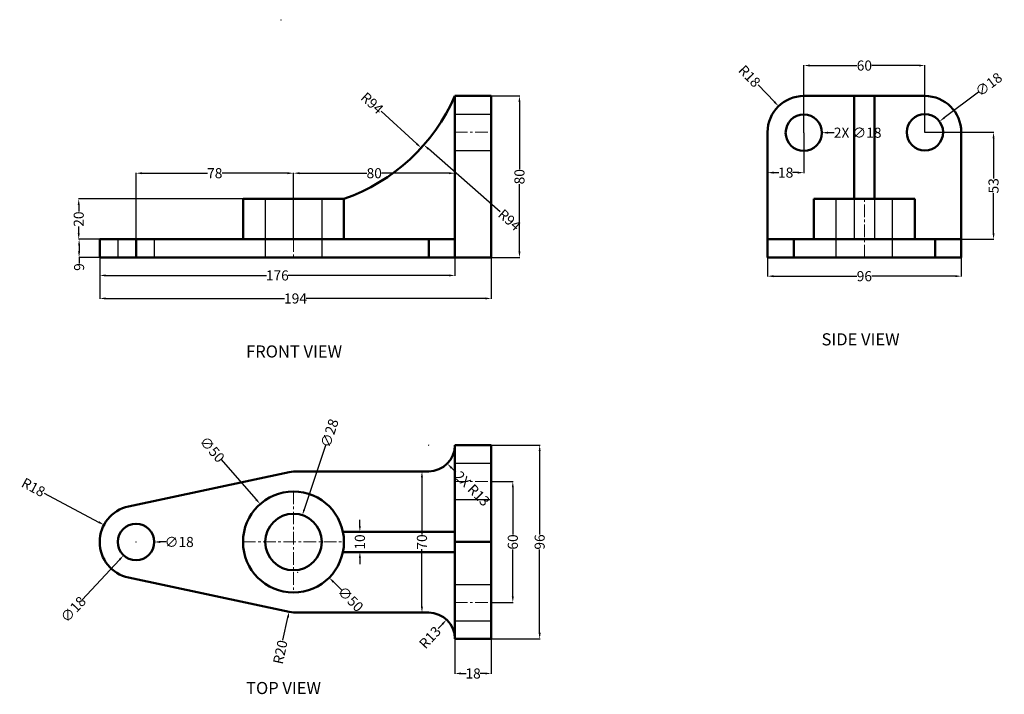
# Model space of a CAD drawing. Units: inches. Extents: x 93 to 580, y -115 to 220.
import ezdxf

# ---------------------------------------------------------------- set-up
doc = ezdxf.new("R2010")
doc.units = ezdxf.units.IN
doc.header["$MEASUREMENT"] = 0
doc.linetypes.add('CENTER', pattern=[2, 1.25, -0.25, 0.25, -0.25])
doc.linetypes.add('HIDDEN', pattern=[9.525, 6.35, -3.175])
for name, color, linetype, lineweight in [('M-CNTR', 1, 'CENTER', 18), ('M-DIMS', 2, 'Continuous', 25), ('M-HIDN', 3, 'HIDDEN', 25), ('M-OUTL', 7, 'Continuous', 50), ('M-TEXT', 7, 'Continuous', 25)]:
    doc.layers.add(name, color=color, linetype=linetype, lineweight=lineweight)
doc.styles.get("Standard").update_dxf_attribs({"font": 'arial.ttf'})
doc.dimstyles.get("Standard").update_dxf_attribs({"dimtxt": 5, "dimasz": 3, "dimexe": 0.18, "dimexo": 0.0625, "dimgap": 0.09, "dimtad": 0, "dimdec": 0, "dimzin": 0, "dimdsep": 46, "dimtxsty": 'Standard', "dimcen": 0.09, "dimadec": 0, "dimazin": 0, "dimtfac": 1, "dimtdec": 0, "dimtofl": 0, "dimtmove": 0, "dimatfit": 3, "dimfxl": 1, "dimtolj": 1, "dimtzin": 0, "dimarcsym": 0})

# ---------------------------------------------------------------- blocks, each defined once
blk = doc.blocks.new('*D1')
at = {"layer": 'Defpoints', "color": 0, "transparency": 16777216}
for p in [(326.19, 181.8), (326.19, 101.8), (340.15, 101.8)]:
    blk.add_point(p, dxfattribs=at)
at = {"layer": 'M-DIMS', "color": 0, "lineweight": -2, "transparency": 16777216}
for p, q in [((326.25, 181.8), (340.33, 181.8)), ((340.15, 178.8), (340.15, 145.46)), ((340.15, 104.8), (340.15, 138.13)), ((326.25, 101.8), (340.33, 101.8))]:
    blk.add_line(p, q, dxfattribs=at)
at = {"layer": 'M-DIMS', "color": 0, "transparency": 16777216}
for points in [[(339.65, 178.8), (340.65, 178.8), (340.15, 181.8)], [(339.65, 104.8), (340.65, 104.8), (340.15, 101.8)]]:
    blk.add_solid(points, dxfattribs=at)
at = {"layer": 'M-DIMS', "color": 0, "transparency": 16777216, "insert": (340.15, 141.8), "char_height": 5, "attachment_point": 5, "rotation": 90}
blk.add_mtext('\\A1;80', dxfattribs=at)
blk = doc.blocks.new('*D2')
at = {"layer": 'Defpoints', "color": 0, "transparency": 16777216}
for p in [(132.19, 101.8), (308.19, 101.8), (308.19, 92.89)]:
    blk.add_point(p, dxfattribs=at)
at = {"layer": 'M-DIMS', "color": 0, "lineweight": -2, "transparency": 16777216}
for p, q in [((132.19, 101.73), (132.19, 92.71)), ((308.19, 101.73), (308.19, 92.71)), ((135.19, 92.89), (214.81, 92.89)), ((305.19, 92.89), (225.57, 92.89))]:
    blk.add_line(p, q, dxfattribs=at)
at = {"layer": 'M-DIMS', "color": 0, "transparency": 16777216}
for points in [[(135.19, 93.39), (135.19, 92.39), (132.19, 92.89)], [(305.19, 93.39), (305.19, 92.39), (308.19, 92.89)]]:
    blk.add_solid(points, dxfattribs=at)
at = {"layer": 'M-DIMS', "color": 0, "transparency": 16777216, "insert": (220.19, 92.89), "char_height": 5, "attachment_point": 5}
blk.add_mtext('\\A1;176', dxfattribs=at)
blk = doc.blocks.new('*D3')
at = {"layer": 'Defpoints', "color": 0, "transparency": 16777216}
for p in [(132.19, 101.8), (326.19, 101.8), (326.19, 81.49)]:
    blk.add_point(p, dxfattribs=at)
at = {"layer": 'M-DIMS', "color": 0, "lineweight": -2, "transparency": 16777216}
for p, q in [((132.19, 101.73), (132.19, 81.31)), ((326.19, 101.73), (326.19, 81.31)), ((135.19, 81.49), (223.82, 81.49)), ((323.19, 81.49), (234.56, 81.49))]:
    blk.add_line(p, q, dxfattribs=at)
at = {"layer": 'M-DIMS', "color": 0, "transparency": 16777216}
for points in [[(135.19, 81.99), (135.19, 80.99), (132.19, 81.49)], [(323.19, 81.99), (323.19, 80.99), (326.19, 81.49)]]:
    blk.add_solid(points, dxfattribs=at)
at = {"layer": 'M-DIMS', "color": 0, "transparency": 16777216, "insert": (229.19, 81.49), "char_height": 5, "attachment_point": 5}
blk.add_mtext('\\A1;194', dxfattribs=at)
blk = doc.blocks.new('*D4')
at = {"layer": 'Defpoints', "color": 0, "transparency": 16777216}
for p in [(132.19, 110.8), (121.98, 101.8), (132.19, 101.8)]:
    blk.add_point(p, dxfattribs=at)
at = {"layer": 'M-DIMS', "color": 0, "lineweight": -2, "transparency": 16777216}
for p, q in [((132.13, 110.8), (121.8, 110.8)), ((121.98, 107.8), (121.98, 104.8)), ((132.13, 101.8), (121.8, 101.8)), ((121.98, 101.8), (121.98, 98.8))]:
    blk.add_line(p, q, dxfattribs=at)
at = {"layer": 'M-DIMS', "color": 0, "transparency": 16777216}
for points in [[(121.48, 107.8), (122.48, 107.8), (121.98, 110.8)], [(121.48, 104.8), (122.48, 104.8), (121.98, 101.8)]]:
    blk.add_solid(points, dxfattribs=at)
at = {"layer": 'M-DIMS', "color": 0, "transparency": 16777216, "insert": (121.98, 97.06), "char_height": 5, "attachment_point": 5, "rotation": 90}
blk.add_mtext('\\A1;9', dxfattribs=at)
blk = doc.blocks.new('*D5')
at = {"layer": 'Defpoints', "color": 0, "transparency": 16777216}
for p in [(121.8, 130.8), (203.19, 130.8), (203.19, 110.8)]:
    blk.add_point(p, dxfattribs=at)
at = {"layer": 'M-DIMS', "color": 0, "lineweight": -2, "transparency": 16777216}
for p, q in [((203.13, 130.8), (121.62, 130.8)), ((121.8, 127.8), (121.8, 124.5)), ((121.8, 113.8), (121.8, 117.09)), ((203.13, 110.8), (121.62, 110.8))]:
    blk.add_line(p, q, dxfattribs=at)
at = {"layer": 'M-DIMS', "color": 0, "transparency": 16777216}
for points in [[(121.3, 127.8), (122.3, 127.8), (121.8, 130.8)], [(121.3, 113.8), (122.3, 113.8), (121.8, 110.8)]]:
    blk.add_solid(points, dxfattribs=at)
at = {"layer": 'M-DIMS', "color": 0, "transparency": 16777216, "insert": (121.8, 120.8), "char_height": 5, "attachment_point": 5, "rotation": 90}
blk.add_mtext('\\A1;20', dxfattribs=at)
blk = doc.blocks.new('*D6')
at = {"layer": 'Defpoints', "color": 0, "transparency": 16777216}
for p in [(228.19, 143.54), (150.19, 110.8), (228.19, 110.8)]:
    blk.add_point(p, dxfattribs=at)
at = {"layer": 'M-DIMS', "color": 0, "lineweight": -2, "transparency": 16777216}
for p, q in [((150.19, 110.86), (150.19, 143.72)), ((153.19, 143.54), (185.53, 143.54)), ((225.19, 143.54), (192.85, 143.54)), ((228.19, 110.86), (228.19, 143.72))]:
    blk.add_line(p, q, dxfattribs=at)
at = {"layer": 'M-DIMS', "color": 0, "transparency": 16777216}
for points in [[(153.19, 144.04), (153.19, 143.04), (150.19, 143.54)], [(225.19, 144.04), (225.19, 143.04), (228.19, 143.54)]]:
    blk.add_solid(points, dxfattribs=at)
at = {"layer": 'M-DIMS', "color": 0, "transparency": 16777216, "insert": (189.19, 143.54), "char_height": 5, "attachment_point": 5}
blk.add_mtext('\\A1;78', dxfattribs=at)
blk = doc.blocks.new('*D7')
at = {"layer": 'Defpoints', "color": 0, "transparency": 16777216}
for p in [(308.19, 143.54), (228.19, 110.8), (308.19, 110.8)]:
    blk.add_point(p, dxfattribs=at)
at = {"layer": 'M-DIMS', "color": 0, "lineweight": -2, "transparency": 16777216}
for p, q in [((228.19, 110.86), (228.19, 143.72)), ((231.19, 143.54), (264.52, 143.54)), ((305.19, 143.54), (271.86, 143.54)), ((308.19, 110.86), (308.19, 143.72))]:
    blk.add_line(p, q, dxfattribs=at)
at = {"layer": 'M-DIMS', "color": 0, "transparency": 16777216}
for points in [[(231.19, 144.04), (231.19, 143.04), (228.19, 143.54)], [(305.19, 144.04), (305.19, 143.04), (308.19, 143.54)]]:
    blk.add_solid(points, dxfattribs=at)
at = {"layer": 'M-DIMS', "color": 0, "transparency": 16777216, "insert": (268.19, 143.54), "char_height": 5, "attachment_point": 5}
blk.add_mtext('\\A1;80', dxfattribs=at)
blk = doc.blocks.new('*D8')
at = {"layer": 'Defpoints', "color": 0, "transparency": 16777216}
for p in [(222.08, 219.5), (291.46, 156.08)]:
    blk.add_point(p, dxfattribs=at)
at = {"layer": 'M-DIMS', "color": 0, "lineweight": -2, "transparency": 16777216}
blk.add_line((271.63, 174.21), (289.25, 158.1), dxfattribs=at)
at = {"layer": 'M-DIMS', "color": 0, "transparency": 16777216}
blk.add_solid([(289.59, 158.47), (288.91, 157.73), (291.46, 156.08)], dxfattribs=at)
at = {"layer": 'M-DIMS', "color": 0, "transparency": 16777216, "insert": (267.16, 178.29), "char_height": 5, "attachment_point": 5, "rotation": 317.5675}
blk.add_mtext('\\A1;R94', dxfattribs=at)
blk = doc.blocks.new('*D9')
at = {"layer": 'Defpoints', "color": 0, "transparency": 16777216}
for p in [(541.03, 196.88), (481.03, 163.61), (541.03, 163.8)]:
    blk.add_point(p, dxfattribs=at)
at = {"layer": 'M-DIMS', "color": 0, "lineweight": -2, "transparency": 16777216}
for p, q in [((481.03, 163.67), (481.03, 197.06)), ((484.03, 196.88), (507.36, 196.88)), ((538.03, 196.88), (514.71, 196.88)), ((541.03, 163.86), (541.03, 197.06))]:
    blk.add_line(p, q, dxfattribs=at)
at = {"layer": 'M-DIMS', "color": 0, "transparency": 16777216}
for points in [[(484.03, 197.38), (484.03, 196.38), (481.03, 196.88)], [(538.03, 197.38), (538.03, 196.38), (541.03, 196.88)]]:
    blk.add_solid(points, dxfattribs=at)
at = {"layer": 'M-DIMS', "color": 0, "transparency": 16777216, "insert": (511.03, 196.88), "char_height": 5, "attachment_point": 5}
blk.add_mtext('\\A1;60', dxfattribs=at)
blk = doc.blocks.new('*D10')
at = {"layer": 'Defpoints', "color": 0, "transparency": 16777216}
for p in [(463.03, 101.8), (559.03, 101.8), (559.03, 92.53)]:
    blk.add_point(p, dxfattribs=at)
at = {"layer": 'M-DIMS', "color": 0, "lineweight": -2, "transparency": 16777216}
for p, q in [((463.03, 101.73), (463.03, 92.35)), ((559.03, 101.73), (559.03, 92.35)), ((466.03, 92.53), (507.36, 92.53)), ((556.03, 92.53), (514.7, 92.53))]:
    blk.add_line(p, q, dxfattribs=at)
at = {"layer": 'M-DIMS', "color": 0, "transparency": 16777216}
for points in [[(466.03, 93.03), (466.03, 92.03), (463.03, 92.53)], [(556.03, 93.03), (556.03, 92.03), (559.03, 92.53)]]:
    blk.add_solid(points, dxfattribs=at)
at = {"layer": 'M-DIMS', "color": 0, "transparency": 16777216, "insert": (511.03, 92.53), "char_height": 5, "attachment_point": 5}
blk.add_mtext('\\A1;96', dxfattribs=at)
blk = doc.blocks.new('*D11')
at = {"layer": 'Defpoints', "color": 0, "transparency": 16777216}
for p in [(541.03, 163.8), (575.03, 163.8), (559.03, 110.8)]:
    blk.add_point(p, dxfattribs=at)
at = {"layer": 'M-DIMS', "color": 0, "lineweight": -2, "transparency": 16777216}
for p, q in [((541.09, 163.8), (575.21, 163.8)), ((575.03, 160.8), (575.03, 140.97)), ((575.03, 113.8), (575.03, 133.63)), ((559.09, 110.8), (575.21, 110.8))]:
    blk.add_line(p, q, dxfattribs=at)
at = {"layer": 'M-DIMS', "color": 0, "transparency": 16777216}
for points in [[(574.53, 160.8), (575.53, 160.8), (575.03, 163.8)], [(574.53, 113.8), (575.53, 113.8), (575.03, 110.8)]]:
    blk.add_solid(points, dxfattribs=at)
at = {"layer": 'M-DIMS', "color": 0, "transparency": 16777216, "insert": (575.03, 137.3), "char_height": 5, "attachment_point": 5, "rotation": 90}
blk.add_mtext('\\A1;53', dxfattribs=at)
blk = doc.blocks.new('*D12')
at = {"layer": 'Defpoints', "color": 0, "transparency": 16777216}
for p in [(463.03, 163.8), (481.03, 163.61), (481.03, 143.82)]:
    blk.add_point(p, dxfattribs=at)
at = {"layer": 'M-DIMS', "color": 0, "lineweight": -2, "transparency": 16777216}
for p, q in [((463.03, 163.73), (463.03, 143.64)), ((481.03, 163.55), (481.03, 143.64)), ((466.03, 143.82), (468.59, 143.82)), ((478.03, 143.82), (475.47, 143.82))]:
    blk.add_line(p, q, dxfattribs=at)
at = {"layer": 'M-DIMS', "color": 0, "transparency": 16777216}
for points in [[(466.03, 144.32), (466.03, 143.32), (463.03, 143.82)], [(478.03, 144.32), (478.03, 143.32), (481.03, 143.82)]]:
    blk.add_solid(points, dxfattribs=at)
at = {"layer": 'M-DIMS', "color": 0, "transparency": 16777216, "insert": (472.03, 143.82), "char_height": 5, "attachment_point": 5}
blk.add_mtext('\\A1;18', dxfattribs=at)
blk = doc.blocks.new('*D13')
at = {"layer": 'Defpoints', "color": 0, "transparency": 16777216}
for p in [(468.52, 176.74), (481.03, 163.8)]:
    blk.add_point(p, dxfattribs=at)
at = {"layer": 'M-DIMS', "color": 0, "lineweight": -2, "transparency": 16777216}
for p, q in [((458.36, 187.26), (466.44, 178.9)), ((480.94, 163.8), (481.12, 163.8)), ((481.03, 163.71), (481.03, 163.89))]:
    blk.add_line(p, q, dxfattribs=at)
at = {"layer": 'M-DIMS', "color": 0, "transparency": 16777216}
blk.add_solid([(466.8, 179.24), (466.08, 178.55), (468.52, 176.74)], dxfattribs=at)
at = {"layer": 'M-DIMS', "color": 0, "transparency": 16777216, "insert": (454.14, 191.62), "char_height": 5, "attachment_point": 5, "rotation": 314.0265}
blk.add_mtext('\\A1;R18', dxfattribs=at)
blk = doc.blocks.new('*D14')
at = {"layer": 'Defpoints', "color": 0, "transparency": 16777216}
for p in [(548.23, 169.2), (533.84, 158.39)]:
    blk.add_point(p, dxfattribs=at)
at = {"layer": 'M-DIMS', "color": 0, "lineweight": -2, "transparency": 16777216}
for p, q in [((567.52, 183.69), (550.63, 171)), ((540.94, 163.8), (541.12, 163.8)), ((541.03, 163.71), (541.03, 163.89))]:
    blk.add_line(p, q, dxfattribs=at)
at = {"layer": 'M-DIMS', "color": 0, "transparency": 16777216}
blk.add_solid([(550.33, 171.4), (550.93, 170.6), (548.23, 169.2)], dxfattribs=at)
at = {"layer": 'M-DIMS', "color": 0, "transparency": 16777216, "insert": (572.64, 187.53), "char_height": 5, "attachment_point": 5, "rotation": 36.9071}
blk.add_mtext('\\A1;∅18', dxfattribs=at)
blk = doc.blocks.new('*D15')
at = {"layer": 'Defpoints', "color": 0, "transparency": 16777216}
for p in [(134.3, -30.69), (150.19, -39.15)]:
    blk.add_point(p, dxfattribs=at)
at = {"layer": 'M-DIMS', "color": 0, "lineweight": -2, "transparency": 16777216}
for p, q in [((104.7, -14.91), (131.66, -29.28)), ((150.1, -39.15), (150.28, -39.15)), ((150.19, -39.24), (150.19, -39.06))]:
    blk.add_line(p, q, dxfattribs=at)
at = {"layer": 'M-DIMS', "color": 0, "transparency": 16777216}
blk.add_solid([(131.89, -28.83), (131.42, -29.72), (134.3, -30.69)], dxfattribs=at)
at = {"layer": 'M-DIMS', "color": 0, "transparency": 16777216, "insert": (99.35, -12.06), "char_height": 5, "attachment_point": 5, "rotation": 331.9512}
blk.add_mtext('\\A1;R18', dxfattribs=at)
blk = doc.blocks.new('*D16')
at = {"layer": 'Defpoints', "color": 0, "transparency": 16777216}
for p in [(156.33, -32.57), (144.05, -45.73)]:
    blk.add_point(p, dxfattribs=at)
at = {"layer": 'M-DIMS', "color": 0, "lineweight": -2, "transparency": 16777216}
for p, q in [((150.1, -39.15), (150.28, -39.15)), ((150.19, -39.24), (150.19, -39.06)), ((123.44, -67.84), (142.01, -47.93))]:
    blk.add_line(p, q, dxfattribs=at)
at = {"layer": 'M-DIMS', "color": 0, "transparency": 16777216}
blk.add_solid([(141.64, -47.59), (142.37, -48.27), (144.05, -45.73)], dxfattribs=at)
at = {"layer": 'M-DIMS', "color": 0, "transparency": 16777216, "insert": (119.07, -72.52), "char_height": 5, "attachment_point": 5, "rotation": 46.9988}
blk.add_mtext('\\A1;∅18', dxfattribs=at)
blk = doc.blocks.new('*D17')
at = {"layer": 'Defpoints', "color": 0, "transparency": 16777216}
for p in [(211.7, -20.36), (244.68, -57.94)]:
    blk.add_point(p, dxfattribs=at)
at = {"layer": 'M-DIMS', "color": 0, "lineweight": -2, "transparency": 16777216}
for p, q in [((192.15, 1.9), (209.72, -18.11)), ((228.1, -39.15), (228.28, -39.15)), ((228.19, -39.24), (228.19, -39.06))]:
    blk.add_line(p, q, dxfattribs=at)
at = {"layer": 'M-DIMS', "color": 0, "transparency": 16777216}
blk.add_solid([(210.1, -17.78), (209.34, -18.44), (211.7, -20.36)], dxfattribs=at)
at = {"layer": 'M-DIMS', "color": 0, "transparency": 16777216, "insert": (187.94, 6.7), "char_height": 5, "attachment_point": 5, "rotation": 311.2749}
blk.add_mtext('\\A1;∅50', dxfattribs=at)
blk = doc.blocks.new('*D18')
at = {"layer": 'Defpoints', "color": 0, "transparency": 16777216}
for p in [(232.59, -25.86), (223.79, -52.44)]:
    blk.add_point(p, dxfattribs=at)
at = {"layer": 'M-DIMS', "color": 0, "lineweight": -2, "transparency": 16777216}
for p, q in [((244.04, 8.67), (233.54, -23.01)), ((228.1, -39.15), (228.28, -39.15)), ((228.19, -39.24), (228.19, -39.06))]:
    blk.add_line(p, q, dxfattribs=at)
at = {"layer": 'M-DIMS', "color": 0, "transparency": 16777216}
blk.add_solid([(233.06, -22.86), (234.01, -23.17), (232.59, -25.86)], dxfattribs=at)
at = {"layer": 'M-DIMS', "color": 0, "transparency": 16777216, "insert": (246.05, 14.75), "char_height": 5, "attachment_point": 5, "rotation": 71.6656}
blk.add_mtext('\\A1;∅28', dxfattribs=at)
blk = doc.blocks.new('*D19')
at = {"layer": 'Defpoints', "color": 0, "transparency": 16777216}
for p in [(230.29, -54.15), (226.03, -73.69)]:
    blk.add_point(p, dxfattribs=at)
at = {"layer": 'M-DIMS', "color": 0, "lineweight": -2, "transparency": 16777216}
for p, q in [((230.2, -54.15), (230.38, -54.15)), ((230.29, -54.24), (230.29, -54.06)), ((222.95, -87.78), (225.39, -76.62))]:
    blk.add_line(p, q, dxfattribs=at)
blk.add_arc((230.29, -54.15), 20, 257.165, 257.8086, dxfattribs=at)
at = {"layer": 'M-DIMS', "color": 0, "transparency": 16777216}
blk.add_solid([(224.9, -76.51), (225.88, -76.73), (226.03, -73.69)], dxfattribs=at)
at = {"layer": 'M-DIMS', "color": 0, "transparency": 16777216, "insert": (221.66, -93.7), "char_height": 5, "attachment_point": 5, "rotation": 77.6807}
blk.add_mtext('\\A1;R20', dxfattribs=at)
blk = doc.blocks.new('*D20')
at = {"layer": 'Defpoints', "color": 0, "transparency": 16777216}
for p in [(265.36, -34.15), (261.09, -44.15), (265.36, -44.15)]:
    blk.add_point(p, dxfattribs=at)
at = {"layer": 'M-DIMS', "color": 0, "lineweight": -2, "transparency": 16777216}
for p, q in [((261.09, -31.15), (261.09, -28.15)), ((265.3, -34.15), (260.91, -34.15)), ((265.3, -44.15), (260.91, -44.15)), ((261.09, -47.15), (261.09, -50.15))]:
    blk.add_line(p, q, dxfattribs=at)
at = {"layer": 'M-DIMS', "color": 0, "transparency": 16777216}
for points in [[(260.59, -31.15), (261.59, -31.15), (261.09, -34.15)], [(260.59, -47.15), (261.59, -47.15), (261.09, -44.15)]]:
    blk.add_solid(points, dxfattribs=at)
at = {"layer": 'M-DIMS', "color": 0, "transparency": 16777216, "insert": (261.09, -39.15), "char_height": 5, "attachment_point": 5, "rotation": 90}
blk.add_mtext('\\A1;10', dxfattribs=at)
blk = doc.blocks.new('*D21')
at = {"layer": 'Defpoints', "color": 0, "transparency": 16777216}
for p in [(295.19, -4.15), (291.84, -74.15), (295.19, -74.15)]:
    blk.add_point(p, dxfattribs=at)
at = {"layer": 'M-DIMS', "color": 0, "lineweight": -2, "transparency": 16777216}
for p, q in [((295.13, -4.15), (291.66, -4.15)), ((291.84, -7.15), (291.84, -35.51)), ((291.84, -71.15), (291.84, -42.79)), ((295.13, -74.15), (291.66, -74.15))]:
    blk.add_line(p, q, dxfattribs=at)
at = {"layer": 'M-DIMS', "color": 0, "transparency": 16777216}
for points in [[(291.34, -7.15), (292.34, -7.15), (291.84, -4.15)], [(291.34, -71.15), (292.34, -71.15), (291.84, -74.15)]]:
    blk.add_solid(points, dxfattribs=at)
at = {"layer": 'M-DIMS', "color": 0, "transparency": 16777216, "insert": (291.84, -39.15), "char_height": 5, "attachment_point": 5, "rotation": 90}
blk.add_mtext('\\A1;70', dxfattribs=at)
blk = doc.blocks.new('*D22')
at = {"layer": 'Defpoints', "color": 0, "transparency": 16777216}
for p in [(304.03, -77.62), (295.19, -87.15)]:
    blk.add_point(p, dxfattribs=at)
at = {"layer": 'M-DIMS', "color": 0, "lineweight": -2, "transparency": 16777216}
blk.add_line((299.95, -82.02), (301.99, -79.82), dxfattribs=at)
at = {"layer": 'M-DIMS', "color": 0, "transparency": 16777216}
blk.add_solid([(301.62, -79.48), (302.36, -80.16), (304.03, -77.62)], dxfattribs=at)
at = {"layer": 'M-DIMS', "color": 0, "transparency": 16777216, "insert": (295.83, -86.46), "char_height": 5, "attachment_point": 5, "rotation": 47.1582}
blk.add_mtext('\\A1;R13', dxfattribs=at)
blk = doc.blocks.new('*D23')
at = {"layer": 'Defpoints', "color": 0, "transparency": 16777216}
for p in [(326.19, -9.15), (326.19, -69.15), (336.86, -69.15)]:
    blk.add_point(p, dxfattribs=at)
at = {"layer": 'M-DIMS', "color": 0, "lineweight": -2, "transparency": 16777216}
for p, q in [((326.25, -9.15), (337.04, -9.15)), ((336.86, -12.15), (336.86, -35.47)), ((336.86, -66.15), (336.86, -42.83)), ((326.25, -69.15), (337.04, -69.15))]:
    blk.add_line(p, q, dxfattribs=at)
at = {"layer": 'M-DIMS', "color": 0, "transparency": 16777216}
for points in [[(336.36, -12.15), (337.36, -12.15), (336.86, -9.15)], [(336.36, -66.15), (337.36, -66.15), (336.86, -69.15)]]:
    blk.add_solid(points, dxfattribs=at)
at = {"layer": 'M-DIMS', "color": 0, "transparency": 16777216, "insert": (336.86, -39.15), "char_height": 5, "attachment_point": 5, "rotation": 90}
blk.add_mtext('\\A1;60', dxfattribs=at)
blk = doc.blocks.new('*D24')
at = {"layer": 'Defpoints', "color": 0, "transparency": 16777216}
for p in [(326.19, 8.85), (326.19, -87.15), (350.16, -87.15)]:
    blk.add_point(p, dxfattribs=at)
at = {"layer": 'M-DIMS', "color": 0, "lineweight": -2, "transparency": 16777216}
for p, q in [((326.25, 8.85), (350.34, 8.85)), ((350.16, 5.85), (350.16, -35.48)), ((350.16, -84.15), (350.16, -42.82)), ((326.25, -87.15), (350.34, -87.15))]:
    blk.add_line(p, q, dxfattribs=at)
at = {"layer": 'M-DIMS', "color": 0, "transparency": 16777216}
for points in [[(349.66, 5.85), (350.66, 5.85), (350.16, 8.85)], [(349.66, -84.15), (350.66, -84.15), (350.16, -87.15)]]:
    blk.add_solid(points, dxfattribs=at)
at = {"layer": 'M-DIMS', "color": 0, "transparency": 16777216, "insert": (350.16, -39.15), "char_height": 5, "attachment_point": 5, "rotation": 90}
blk.add_mtext('\\A1;96', dxfattribs=at)
blk = doc.blocks.new('*D25')
at = {"layer": 'Defpoints', "color": 0, "transparency": 16777216}
for p in [(308.19, -87.15), (326.19, -87.15), (326.19, -104.29)]:
    blk.add_point(p, dxfattribs=at)
at = {"layer": 'M-DIMS', "color": 0, "lineweight": -2, "transparency": 16777216}
for p, q in [((308.19, -87.21), (308.19, -104.47)), ((326.19, -87.21), (326.19, -104.47)), ((311.19, -104.29), (313.75, -104.29)), ((323.19, -104.29), (320.63, -104.29))]:
    blk.add_line(p, q, dxfattribs=at)
at = {"layer": 'M-DIMS', "color": 0, "transparency": 16777216}
for points in [[(311.19, -103.79), (311.19, -104.79), (308.19, -104.29)], [(323.19, -103.79), (323.19, -104.79), (326.19, -104.29)]]:
    blk.add_solid(points, dxfattribs=at)
at = {"layer": 'M-DIMS', "color": 0, "transparency": 16777216, "insert": (317.19, -104.29), "char_height": 5, "attachment_point": 5}
blk.add_mtext('\\A1;18', dxfattribs=at)
blk = doc.blocks.new('*D26')
at = {"layer": 'Defpoints', "color": 0, "transparency": 16777216}
for p in [(222.08, 219.5), (292.79, 157.56)]:
    blk.add_point(p, dxfattribs=at)
at = {"layer": 'M-DIMS', "color": 0, "lineweight": -2, "transparency": 16777216}
for p, q in [((222.08, 219.41), (222.08, 219.59)), ((221.99, 219.5), (222.17, 219.5)), ((330.66, 124.38), (295.04, 155.58))]:
    blk.add_line(p, q, dxfattribs=at)
at = {"layer": 'M-DIMS', "color": 0, "transparency": 16777216}
blk.add_solid([(295.37, 155.96), (294.71, 155.2), (292.79, 157.56)], dxfattribs=at)
at = {"layer": 'M-DIMS', "color": 0, "transparency": 16777216, "insert": (335.21, 120.39), "char_height": 5, "attachment_point": 5, "rotation": 318.7788}
blk.add_mtext('\\A1;R94', dxfattribs=at)
blk = doc.blocks.new('*D27')
at = {"layer": 'Defpoints', "color": 0, "transparency": 16777216}
for p in [(472.03, 163.61), (490.03, 163.61)]:
    blk.add_point(p, dxfattribs=at)
at = {"layer": 'M-DIMS', "color": 0, "lineweight": -2, "transparency": 16777216}
for p, q in [((480.94, 163.61), (481.12, 163.61)), ((481.03, 163.52), (481.03, 163.7)), ((496.03, 163.61), (493.03, 163.61))]:
    blk.add_line(p, q, dxfattribs=at)
at = {"layer": 'M-DIMS', "color": 0, "transparency": 16777216}
blk.add_solid([(493.03, 164.11), (493.03, 163.11), (490.03, 163.61)], dxfattribs=at)
at = {"layer": 'M-DIMS', "color": 0, "transparency": 16777216, "insert": (507.71, 163.61), "char_height": 5, "attachment_point": 5, "rotation": 359.9976}
blk.add_mtext('\\A1;2X ∅18', dxfattribs=at)
blk = doc.blocks.new('*D28')
at = {"layer": 'Defpoints', "color": 0, "transparency": 16777216}
for p in [(141.19, -39.15), (159.19, -39.15)]:
    blk.add_point(p, dxfattribs=at)
at = {"layer": 'M-DIMS', "color": 0, "lineweight": -2, "transparency": 16777216}
for p, q in [((150.1, -39.15), (150.28, -39.15)), ((150.19, -39.24), (150.19, -39.06)), ((165.19, -39.15), (162.19, -39.15))]:
    blk.add_line(p, q, dxfattribs=at)
at = {"layer": 'M-DIMS', "color": 0, "transparency": 16777216}
blk.add_solid([(162.19, -38.65), (162.19, -39.65), (159.19, -39.15)], dxfattribs=at)
at = {"layer": 'M-DIMS', "color": 0, "transparency": 16777216, "insert": (171.59, -39.15), "char_height": 5, "attachment_point": 5, "rotation": 0.0008}
blk.add_mtext('\\A1;∅18', dxfattribs=at)
blk = doc.blocks.new('*D29')
at = {"layer": 'Defpoints', "color": 0, "transparency": 16777216}
for p in [(210.51, -21.47), (245.87, -56.83)]:
    blk.add_point(p, dxfattribs=at)
at = {"layer": 'M-DIMS', "color": 0, "lineweight": -2, "transparency": 16777216}
for p, q in [((228.1, -39.15), (228.28, -39.15)), ((228.19, -39.24), (228.19, -39.06)), ((251.96, -62.92), (247.99, -58.95))]:
    blk.add_line(p, q, dxfattribs=at)
at = {"layer": 'M-DIMS', "color": 0, "transparency": 16777216}
blk.add_solid([(248.34, -58.6), (247.64, -59.3), (245.87, -56.83)], dxfattribs=at)
at = {"layer": 'M-DIMS', "color": 0, "transparency": 16777216, "insert": (256.47, -67.43), "char_height": 5, "attachment_point": 5, "rotation": 314.9994}
blk.add_mtext('\\A1;∅50', dxfattribs=at)
blk = doc.blocks.new('*D30')
at = {"layer": 'Defpoints', "color": 0, "transparency": 16777216}
for p in [(295.19, 8.85), (304.38, -0.34)]:
    blk.add_point(p, dxfattribs=at)
at = {"layer": 'M-DIMS', "color": 0, "lineweight": -2, "transparency": 16777216}
for p, q in [((295.1, 8.85), (295.28, 8.85)), ((295.19, 8.76), (295.19, 8.94)), ((308.63, -4.59), (306.5, -2.46))]:
    blk.add_line(p, q, dxfattribs=at)
at = {"layer": 'M-DIMS', "color": 0, "transparency": 16777216}
blk.add_solid([(306.86, -2.11), (306.15, -2.82), (304.38, -0.34)], dxfattribs=at)
at = {"layer": 'M-DIMS', "color": 0, "transparency": 16777216, "insert": (316.74, -12.7), "char_height": 5, "attachment_point": 5, "rotation": 314.9988}
blk.add_mtext('\\A1;2X R13', dxfattribs=at)

msp = doc.modelspace()

# ---------------------------------------------------------------- linework, layer by layer
at = {"layer": 'M-CNTR', "ltscale": 5}
for p, q in [((308.19, 163.8), (326.19, 163.8)), ((228.19, 130.8), (228.19, 101.8)), ((511.03, 101.8), (511.03, 130.8)), ((308.19, -9.15), (326.19, -9.15)), ((228.19, -14.15), (228.19, -64.15)), ((203.19, -39.15), (253.19, -39.15)), ((308.19, -69.15), (326.19, -69.15))]:
    msp.add_line(p, q, dxfattribs=at)
at = {"layer": 'M-HIDN', "ltscale": 8}
for p, q in [((308.19, 172.8), (326.19, 172.8)), ((308.19, 154.8), (326.19, 154.8)), ((214.19, 130.8), (214.19, 101.8)), ((242.19, 130.8), (242.19, 101.8)), ((497.03, 101.8), (497.03, 130.8)), ((506.03, 130.8), (506.03, 110.8)), ((516.03, 130.8), (516.03, 110.8)), ((525.03, 101.8), (525.03, 130.8)), ((141.19, 110.8), (141.19, 101.8)), ((159.19, 110.8), (159.19, 101.8)), ((308.19, -0.15), (326.19, -0.15)), ((308.19, -18.15), (326.19, -18.15)), ((308.19, -60.15), (326.19, -60.15)), ((308.19, -78.15), (326.19, -78.15))]:
    msp.add_line(p, q, dxfattribs=at)
at = {"layer": 'M-OUTL'}
for p, q in [((326.19, 181.8), (308.19, 181.8)), ((308.19, 181.8), (308.19, 101.8)), ((326.19, 101.8), (326.19, 181.8)), ((541.03, 181.8), (481.03, 181.8)), ((506.03, 130.8), (506.03, 181.8)), ((516.03, 130.8), (516.03, 181.8)), ((463.03, 163.8), (463.03, 101.8)), ((559.03, 101.8), (559.03, 163.8)), ((203.19, 130.8), (253.19, 130.8)), ((203.19, 130.8), (203.19, 110.8)), ((253.19, 130.8), (253.19, 110.8)), ((486.03, 130.8), (536.03, 130.8)), ((486.03, 110.8), (486.03, 130.8)), ((536.03, 110.8), (536.03, 130.8)), ((132.19, 110.8), (308.19, 110.8)), ((132.19, 110.8), (132.19, 101.8)), ((150.19, 110.8), (150.19, 101.8)), ((295.19, 110.8), (295.19, 101.8)), ((463.03, 110.8), (559.03, 110.8)), ((476.03, 110.8), (476.03, 101.8)), ((546.03, 101.8), (546.03, 110.8)), ((132.19, 101.8), (326.19, 101.8)), ((463.03, 101.8), (559.03, 101.8)), ((308.19, 8.85), (308.19, -87.15)), ((308.19, 8.85), (326.19, 8.85)), ((326.19, 8.85), (326.19, -87.15)), ((146.44, -21.54), (226.13, -4.59)), ((230.29, -4.15), (295.19, -4.15)), ((252.69, -34.15), (308.19, -34.15)), ((308.19, -39.15), (326.19, -39.15)), ((252.69, -44.15), (308.19, -44.15)), ((146.44, -56.76), (226.13, -73.71)), ((230.29, -74.15), (295.19, -74.15)), ((308.19, -87.15), (326.19, -87.15))]:
    msp.add_line(p, q, dxfattribs=at)
for centre, radius in [((481.03, 163.61), 9), ((541.03, 163.8), 9), ((228.19, -39.15), 25), ((228.19, -39.15), 14), ((150.19, -39.15), 9)]:
    msp.add_circle(centre, radius, dxfattribs=at)
for centre, radius, start, end in [((222.08, 219.5), 94, 289.325, 336.3528), ((481.03, 163.8), 18, 90, 180), ((541.03, 163.8), 18, 0, 90), ((295.19, 8.85), 13, 270, 0), ((230.29, -24.15), 20, 90, 102.0124), ((150.19, -39.15), 18, 102.0124, 257.9876), ((230.29, -54.15), 20, 257.9876, 270), ((295.19, -87.15), 13, 0, 90)]:
    msp.add_arc(centre, radius, start, end, dxfattribs=at)

# ---------------------------------------------------------------- texts
at = {"layer": 'M-TEXT', "char_height": 6, "attachment_point": 1}
for s, insert in [('SIDE VIEW', (489.81, 64.24)), ('FRONT VIEW', (204.72, 58.23)), ('TOP VIEW', (204.72, -108.5))]:
    msp.add_mtext_dynamic_manual_height_columns(s, width=76.1598, gutter_width=1, heights=[0], dxfattribs=dict(at, insert=insert))

# ---------------------------------------------------------------- dimensions: what is measured, and where the dimension line sits
at = {"layer": 'M-DIMS'}
for center, mpoint, override, picture, middle in [((222.08, 219.5), (292.79, 157.56), {"dimdec": 0, "dimlfac": 1, "dimrnd": 0, "dimzin": 0, "dimdsep": 46, "dimlunit": 2}, '*D26', (335.21, 120.39)), ((222.08, 219.5), (291.46, 156.08), {"dimclrd": 0, "dimclre": 0, "dimclrt": 0}, '*D8', (267.16, 178.29)), ((481.03, 163.8), (468.52, 176.74), {"dimclrd": 0, "dimclre": 0, "dimclrt": 0}, '*D13', (454.14, 191.62)), ((150.19, -39.15), (134.3, -30.69), {"dimclrd": 0, "dimclre": 0, "dimclrt": 0}, '*D15', (99.35, -12.06)), ((230.29, -54.15), (226.03, -73.69), {"dimclrd": 0, "dimclre": 0, "dimclrt": 0}, '*D19', (221.66, -93.7)), ((295.19, -87.15), (304.03, -77.62), {"dimclrd": 0, "dimclre": 0, "dimclrt": 0}, '*D22', (295.83, -86.46))]:
    dim = msp.add_radius_dim(center=center, mpoint=mpoint, dimstyle='Standard', override=override, dxfattribs=at)
    dim.commit()
    dim.dimension.update_dxf_attribs({"geometry": picture, "text_midpoint": middle, "dimtype": 164})
for base, p1, p2, picture, middle in [((541.03, 196.88), (481.03, 163.61), (541.03, 163.8), '*D9', (511.03, 196.88)), ((481.03, 143.82), (463.03, 163.8), (481.03, 163.61), '*D12', (472.03, 143.82)), ((228.19, 143.54), (150.19, 110.8), (228.19, 110.8), '*D6', (189.19, 143.54)), ((308.19, 143.54), (228.19, 110.8), (308.19, 110.8), '*D7', (268.19, 143.54)), ((308.19, 92.89), (132.19, 101.8), (308.19, 101.8), '*D2', (220.19, 92.89)), ((326.19, 81.49), (132.19, 101.8), (326.19, 101.8), '*D3', (229.19, 81.49)), ((559.03, 92.53), (463.03, 101.8), (559.03, 101.8), '*D10', (511.03, 92.53)), ((326.19, -104.29), (308.19, -87.15), (326.19, -87.15), '*D25', (317.19, -104.29))]:
    dim = msp.add_linear_dim(base=base, p1=p1, p2=p2, dimstyle='Standard', override={"dimclrd": 0, "dimclre": 0, "dimclrt": 0}, dxfattribs=at)
    dim.commit()
    dim.dimension.update_dxf_attribs({"geometry": picture, "text_midpoint": middle})
for p1, p2, override, picture, middle in [((533.84, 158.39), (548.23, 169.2), {"dimclrd": 0, "dimclre": 0, "dimclrt": 0}, '*D14', (572.64, 187.53)), ((223.79, -52.44), (232.59, -25.86), {"dimclrd": 0, "dimclre": 0, "dimclrt": 0}, '*D18', (246.05, 14.75)), ((244.68, -57.94), (211.7, -20.36), {"dimclrd": 0, "dimclre": 0, "dimclrt": 0}, '*D17', (187.94, 6.7)), ((210.51, -21.47), (245.87, -56.83), {"dimdec": 0, "dimlfac": 1, "dimrnd": 0, "dimzin": 0, "dimdsep": 46, "dimlunit": 2}, '*D29', (256.47, -67.43)), ((156.33, -32.57), (144.05, -45.73), {"dimclrd": 0, "dimclre": 0, "dimclrt": 0}, '*D16', (119.07, -72.52)), ((141.19, -39.15), (159.19, -39.15), {"dimdec": 0, "dimlfac": 1, "dimrnd": 0, "dimzin": 0, "dimdsep": 46, "dimlunit": 2}, '*D28', (171.59, -39.15))]:
    dim = msp.add_diameter_dim_2p(p1=p1, p2=p2, dimstyle='Standard', override=override, dxfattribs=at)
    dim.commit()
    dim.dimension.update_dxf_attribs({"geometry": picture, "text_midpoint": middle, "dimtype": 163})
for base, p1, p2, picture, middle in [((340.15, 101.8), (326.19, 181.8), (326.19, 101.8), '*D1', (340.15, 141.8)), ((575.03, 163.8), (559.03, 110.8), (541.03, 163.8), '*D11', (575.03, 137.3)), ((121.8, 130.8), (203.19, 110.8), (203.19, 130.8), '*D5', (121.8, 120.8)), ((121.98, 101.8), (132.19, 110.8), (132.19, 101.8), '*D4', (121.98, 97.06)), ((350.16, -87.15), (326.19, 8.85), (326.19, -87.15), '*D24', (350.16, -39.15)), ((291.84, -74.15), (295.19, -4.15), (295.19, -74.15), '*D21', (291.84, -39.15)), ((336.86, -69.15), (326.19, -9.15), (326.19, -69.15), '*D23', (336.86, -39.15)), ((261.09, -44.15), (265.36, -34.15), (265.36, -44.15), '*D20', (261.09, -39.15))]:
    dim = msp.add_linear_dim(base=base, p1=p1, p2=p2, angle=90, dimstyle='Standard', override={"dimclrd": 0, "dimclre": 0, "dimclrt": 0}, dxfattribs=at)
    dim.commit()
    dim.dimension.update_dxf_attribs({"geometry": picture, "text_midpoint": middle})
dim = msp.add_diameter_dim_2p(p1=(472.03, 163.61), p2=(490.03, 163.61), text='2X <>', dimstyle='Standard', override={"dimdec": 0, "dimlfac": 1, "dimrnd": 0, "dimzin": 0, "dimdsep": 46, "dimlunit": 2}, dxfattribs=at)
dim.commit()
dim.dimension.update_dxf_attribs({"geometry": '*D27', "text_midpoint": (507.71, 163.61), "dimtype": 163})
dim = msp.add_radius_dim(center=(295.19, 8.85), mpoint=(304.38, -0.34), text='2X <>', dimstyle='Standard', override={"dimdec": 0, "dimlfac": 1, "dimrnd": 0, "dimzin": 0, "dimdsep": 46, "dimlunit": 2}, dxfattribs=at)
dim.commit()
dim.dimension.update_dxf_attribs({"geometry": '*D30', "text_midpoint": (316.74, -12.7)})

doc.saveas('drawing.dxf')
